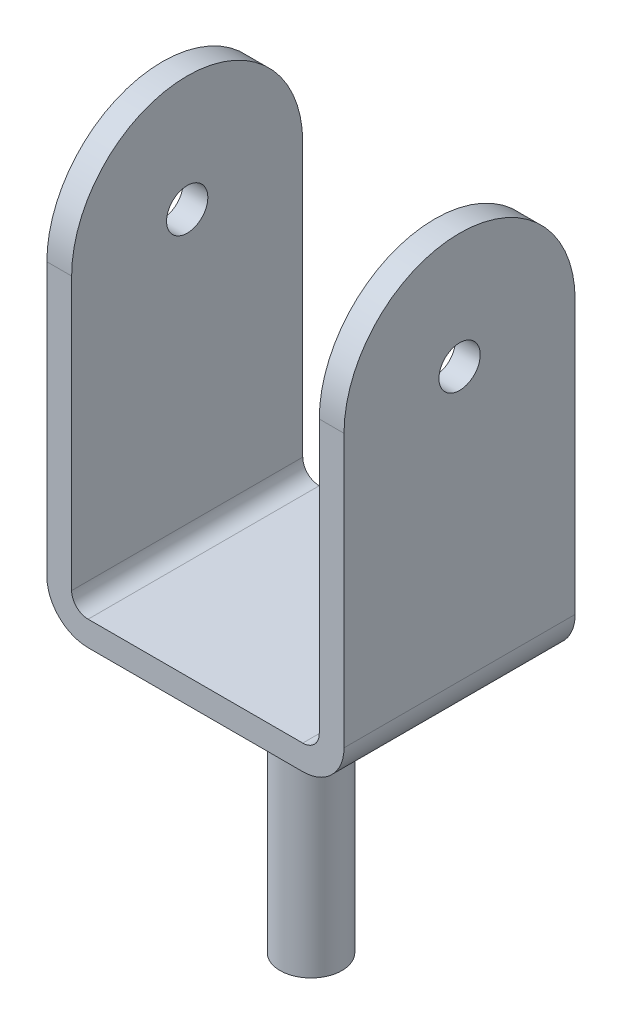
SolidWorks part; units mm, degrees
material "Brass"
ref_plane "Front Plane" through (0, 0, 0) normal (0, 0, 1) x (1, 0, 0)
ref_plane "Top Plane" through (0, 0, 0) normal (0, 1, 0) x (1, 0, 0)
ref_plane "Right Plane" through (0, 0, 0) normal (1, 0, 0) x (0, 0, -1)
sketch "U-Channel Profile Sketch" plane through (0, 0, 0) normal (0, 0, 1) x (1, 0, 0)
  line L0 (-180, 520) -> (-180, 50)
  line L1 (-130, 0) -> (130, 0)
  line L2 (180, 50) -> (180, 520)
  line L3 (180, 520) -> (150, 520)
  line L4 (150, 520) -> (150, 50)
  line L5 (130, 30) -> (-130, 30)
  line L6 (-150, 50) -> (-150, 520)
  line L7 (-150, 520) -> (-180, 520)
  line L8 (0, 0) -> (0, 520) construction
  arc A0 (130, 0) -> (180, 50) centre (130, 50) ccw
  arc A1 (-180, 50) -> (-130, 0) centre (-130, 50) ccw
  arc A2 (150, 50) -> (130, 30) centre (130, 50) cw
  arc A3 (-130, 30) -> (-150, 50) centre (-130, 50) cw
  point P16 (180, 0)
  dimension "D5" = 50
  dimension "D6" = 20
  dimension "D1" = 30
  dimension "D2" = 360
  dimension "D3" = 30
  dimension "D4" = 520
extrude "U-Channel Body" add sketch "U-Channel Profile Sketch" along normal mid plane 280
sketch "Rounded Ends and Pin Hole Sketch" plane through (0, 0, 0) normal (1, 0, 0) x (0, 0, -1)
  line L0 (-140, 520) -> (140, 520) construction
  line L1 (140, 50) -> (140, 520) construction
  line L3 (-140, 50) -> (-140, 520) construction
  line L4 (-140, 520) -> (140, 520)
  line L5 (140, 380) -> (140, 520)
  line L7 (-140, 380) -> (-140, 520)
  arc A0 (140, 380) -> (-140, 380) centre (0, 380) ccw
  circle A1 centre (0, 380) radius 25
  dimension "D1" = 280
  dimension "D2" = 50
extrude "Rounded Ends and Pin Holes" cut sketch "Rounded Ends and Pin Hole Sketch" against normal through all both and the other way through all contours A0 L4 L7 | A0 L5 L4 | A1
sketch "Shank Profile Sketch" plane through (0, 30, 0) normal (0, 1, 0) x (1, 0, 0)
  circle A0 centre (0, 0) radius 37.5
  dimension "D1" = 75
extrude "Round Shank" add sketch "Shank Profile Sketch" against normal blind 355 contours A0
